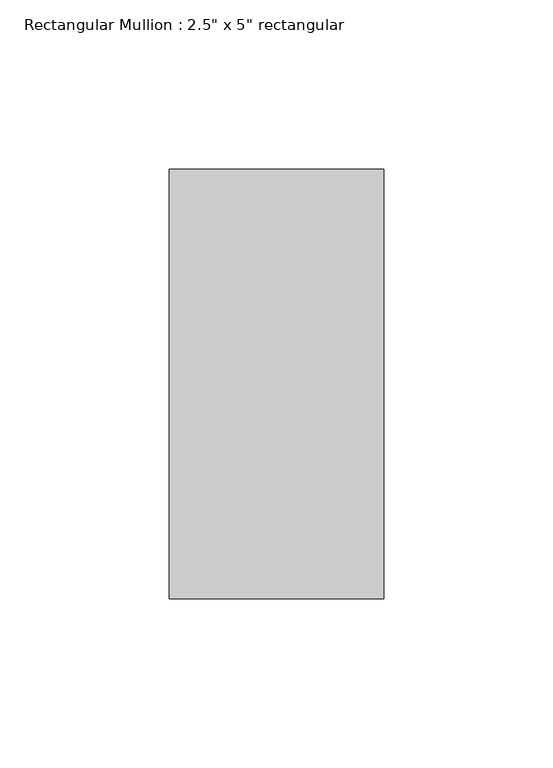
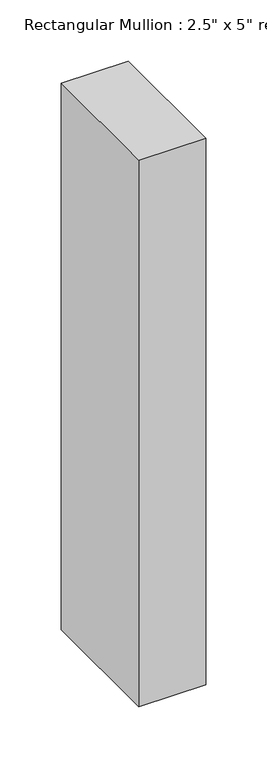
"""IFC4 building model written with IfcOpenShell, lengths in millimetres: member geometry."""

from ifc_helpers import new_model, si_unit, frame, origin, place, context, project, spatial, polyline, outline, extrude, source, transform, mapped, element, save


def member_a980948f(model_context):
    return source(origin(), model_context, "Body", "SweptSolid", [
        extrude(outline(polyline([(0.0, 63.5), (0.0, -63.5), (-63.5, -63.5), (-63.5, 63.5), (0.0, 63.5)])), frame((0.0, 0.0, -546.1), z_axis=(0.0, 0.0, 1.0), x_axis=(1.0, 0.0, 0.0)), (0.0, 0.0, 1.0), 546.1),
    ])


if __name__ == "__main__":
    model = new_model("IFC4")
    model_context = context("Model", 3, world=origin())
    ifc_project = project(units=[si_unit("LENGTHUNIT", "METRE", prefix="MILLI")], contexts=[model_context])
    site = spatial("IfcSite", under=ifc_project)
    building = spatial("IfcBuilding", under=site)
    placement = place(None, origin())
    member_shape = member_a980948f(model_context)
    element("IfcMember", 1, ObjectType="Rectangular Mullion : 2.5\" x 5\" rectangular", at=placement, inside=building, context=model_context, shape_type="MappedRepresentation", body=[
        mapped(member_shape, transform((0.0, 0.0, 0.0), x_axis=(1.0, 0.0, 0.0), y_axis=(0.0, 1.0, 0.0), z_axis=(0.0, 0.0, 1.0))),
    ])
    save(model, "model.ifc")

# Revit data of these elements
# Type "Rectangular Mullion : 2.5\" x 5\" rectangular"
#   built-in parameter 1007304 = 0.416667 (stored number, unit not read)
#   built-in parameter 1007301 = 0.104167 (stored number, unit not read)
#   built-in parameter 1007300 = 0.104167 (stored number, unit not read)
